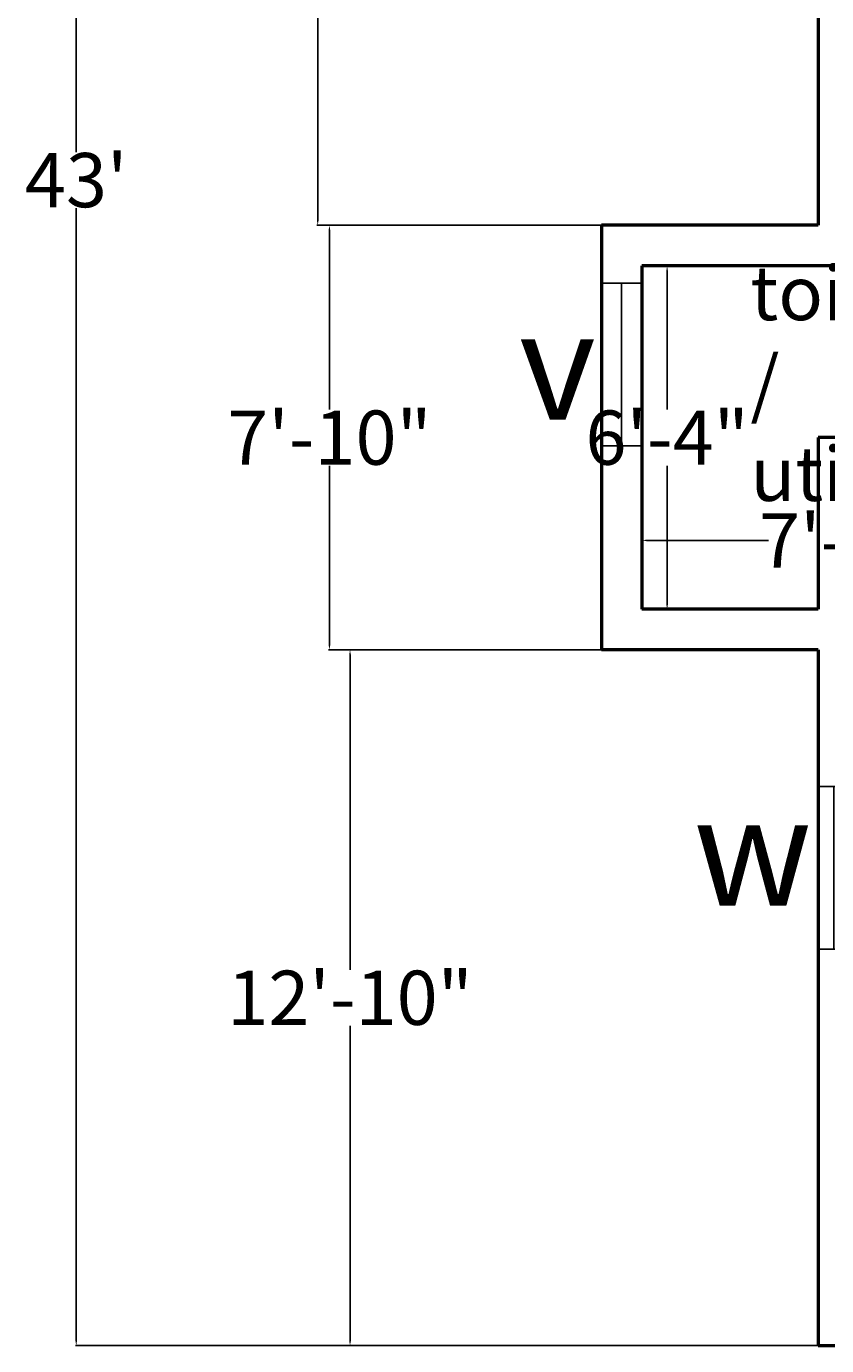
# Model space of a CAD drawing. Units: inches. Extents: x 409 to 7572, y 7 to 725.
# Tile 7 of 38: x 1521 to 1698, y 157 to 449. Entities that reach past the tile are written whole.
import ezdxf

# ---------------------------------------------------------------- set-up
doc = ezdxf.new("R2010")
doc.units = ezdxf.units.IN
doc.header["$MEASUREMENT"] = 0
for name, color, linetype, lineweight in [('A-ANNO-DIMS', 2, 'Continuous', 18), ('A-ANNO-SYMB', 3, 'Continuous', 25), ('A-AREA-IDEN', 7, 'Continuous', 25), ('A-GLAZ', 4, 'Continuous', 25), ('A-WALL', 7, 'Continuous', 50)]:
    doc.layers.add(name, color=color, linetype=linetype, lineweight=lineweight)
doc.styles.get("Standard").update_dxf_attribs({"font": 'arial.ttf'})
doc.dimstyles.get("Standard").update_dxf_attribs({"dimtxt": 2, "dimasz": 1, "dimexe": 0.18, "dimexo": 0.0625, "dimgap": 0.09, "dimtad": 0, "dimtih": 1, "dimtoh": 1, "dimdec": 0, "dimzin": 0, "dimdsep": 46, "dimlunit": 3, "dimtxsty": 'Standard', "dimcen": 0.09, "dimadec": 0, "dimazin": 0, "dimtfac": 1, "dimtdec": 0, "dimtofl": 0, "dimtmove": 0, "dimatfit": 3, "dimfxl": 1, "dimtolj": 1, "dimtzin": 0, "dimarcsym": 0})

# ---------------------------------------------------------------- blocks, each defined once
blk = doc.blocks.new('*D59')
at = {"layer": 'A-ANNO-DIMS', "color": 0, "lineweight": -2, "transparency": 16777216}
for p, q in [((1666.52, 395.53), (1662.7, 395.53)), ((1662.88, 394.53), (1662.88, 363.75)), ((1662.88, 320.53), (1662.88, 351.31)), ((1666.52, 319.53), (1662.7, 319.53))]:
    blk.add_line(p, q, dxfattribs=at)
at = {"layer": 'A-ANNO-DIMS', "color": 0, "transparency": 16777216}
for points in [[(1662.71, 394.53), (1663.05, 394.53), (1662.88, 395.53)], [(1662.71, 320.53), (1663.05, 320.53), (1662.88, 319.53)]]:
    blk.add_solid(points, dxfattribs=at)
at = {"layer": 'DEFPOINTS', "color": 0, "transparency": 16777216}
for p in [(1666.58, 395.53), (1662.88, 319.53), (1666.58, 319.53)]:
    blk.add_point(p, dxfattribs=at)
at = {"layer": 'A-ANNO-DIMS', "color": 0, "transparency": 16777216, "insert": (1662.88, 357.53), "char_height": 2, "attachment_point": 5}
blk.add_mtext('\\A1;{\\H6x;6\'-4"}', dxfattribs=at)
blk = doc.blocks.new('*D61')
at = {"layer": 'A-ANNO-DIMS', "color": 0, "lineweight": -2, "transparency": 16777216}
for p, q in [((1657.32, 346.33), (1657.32, 334.6)), ((1745.32, 346.33), (1745.32, 334.6)), ((1658.32, 334.78), (1685.33, 334.78)), ((1744.32, 334.78), (1717.31, 334.78))]:
    blk.add_line(p, q, dxfattribs=at)
at = {"layer": 'A-ANNO-DIMS', "color": 0, "transparency": 16777216}
for points in [[(1658.32, 334.95), (1658.32, 334.61), (1657.32, 334.78)], [(1744.32, 334.95), (1744.32, 334.61), (1745.32, 334.78)]]:
    blk.add_solid(points, dxfattribs=at)
at = {"layer": 'DEFPOINTS', "color": 0, "transparency": 16777216}
for p in [(1657.32, 346.39), (1745.32, 346.39), (1745.32, 334.78)]:
    blk.add_point(p, dxfattribs=at)
at = {"layer": 'A-ANNO-DIMS', "color": 0, "transparency": 16777216, "insert": (1701.32, 334.78), "char_height": 2, "attachment_point": 5}
blk.add_mtext('\\A1;{\\H6x;7\'-4"}', dxfattribs=at)
blk = doc.blocks.new('*D48')
at = {"layer": 'A-ANNO-DIMS', "color": 0, "lineweight": -2, "transparency": 16777216}
for p, q in [((1696.26, 672.53), (1585.36, 672.53)), ((1585.54, 671.53), (1585.54, 544.65)), ((1585.54, 405.53), (1585.54, 532.42)), ((1696.26, 404.53), (1585.36, 404.53))]:
    blk.add_line(p, q, dxfattribs=at)
at = {"layer": 'A-ANNO-DIMS', "color": 0, "transparency": 16777216}
for points in [[(1585.37, 671.53), (1585.71, 671.53), (1585.54, 672.53)], [(1585.37, 405.53), (1585.71, 405.53), (1585.54, 404.53)]]:
    blk.add_solid(points, dxfattribs=at)
at = {"layer": 'DEFPOINTS', "color": 0, "transparency": 16777216}
for p in [(1696.32, 672.53), (1585.54, 404.53), (1696.32, 404.53)]:
    blk.add_point(p, dxfattribs=at)
at = {"layer": 'A-ANNO-DIMS', "color": 0, "transparency": 16777216, "insert": (1585.54, 538.53), "char_height": 2, "attachment_point": 5}
blk.add_mtext('\\A1;{\\H6x;22\'-4"}', dxfattribs=at)
blk = doc.blocks.new('*D49')
at = {"layer": 'A-ANNO-DIMS', "color": 0, "lineweight": -2, "transparency": 16777216}
for p, q in [((1648.26, 404.53), (1587.95, 404.53)), ((1588.13, 403.53), (1588.13, 363.75)), ((1588.13, 311.53), (1588.13, 351.31)), ((1648.26, 310.53), (1587.95, 310.53))]:
    blk.add_line(p, q, dxfattribs=at)
at = {"layer": 'A-ANNO-DIMS', "color": 0, "transparency": 16777216}
for points in [[(1587.96, 403.53), (1588.29, 403.53), (1588.13, 404.53)], [(1587.96, 311.53), (1588.29, 311.53), (1588.13, 310.53)]]:
    blk.add_solid(points, dxfattribs=at)
at = {"layer": 'DEFPOINTS', "color": 0, "transparency": 16777216}
for p in [(1648.32, 404.53), (1588.13, 310.53), (1648.32, 310.53)]:
    blk.add_point(p, dxfattribs=at)
at = {"layer": 'A-ANNO-DIMS', "color": 0, "transparency": 16777216, "insert": (1588.13, 357.53), "char_height": 2, "attachment_point": 5}
blk.add_mtext('\\A1;{\\H6x;7\'-10"}', dxfattribs=at)
blk = doc.blocks.new('*D50')
at = {"layer": 'A-ANNO-DIMS', "color": 0, "lineweight": -2, "transparency": 16777216}
for p, q in [((1696.26, 310.53), (1592.51, 310.53)), ((1592.69, 309.53), (1592.69, 239.75)), ((1592.69, 157.53), (1592.69, 227.31)), ((1696.26, 156.53), (1592.51, 156.53))]:
    blk.add_line(p, q, dxfattribs=at)
at = {"layer": 'A-ANNO-DIMS', "color": 0, "transparency": 16777216}
for points in [[(1592.52, 309.53), (1592.86, 309.53), (1592.69, 310.53)], [(1592.52, 157.53), (1592.86, 157.53), (1592.69, 156.53)]]:
    blk.add_solid(points, dxfattribs=at)
at = {"layer": 'DEFPOINTS', "color": 0, "transparency": 16777216}
for p in [(1696.32, 310.53), (1592.69, 156.53), (1696.32, 156.53)]:
    blk.add_point(p, dxfattribs=at)
at = {"layer": 'A-ANNO-DIMS', "color": 0, "transparency": 16777216, "insert": (1592.69, 233.53), "char_height": 2, "attachment_point": 5}
blk.add_mtext('\\A1;{\\H6x;12\'-10"}', dxfattribs=at)
blk = doc.blocks.new('*D37')
at = {"layer": 'A-ANNO-DIMS', "color": 0, "lineweight": -2, "transparency": 16777216}
for p, q in [((1696.26, 672.53), (1531.9, 672.53)), ((1532.08, 671.53), (1532.08, 420.75)), ((1532.08, 157.53), (1532.08, 408.31)), ((1696.26, 156.53), (1531.9, 156.53))]:
    blk.add_line(p, q, dxfattribs=at)
at = {"layer": 'A-ANNO-DIMS', "color": 0, "transparency": 16777216}
for points in [[(1531.91, 671.53), (1532.25, 671.53), (1532.08, 672.53)], [(1531.91, 157.53), (1532.25, 157.53), (1532.08, 156.53)]]:
    blk.add_solid(points, dxfattribs=at)
at = {"layer": 'DEFPOINTS', "color": 0, "transparency": 16777216}
for p in [(1696.32, 672.53), (1532.08, 156.53), (1696.32, 156.53)]:
    blk.add_point(p, dxfattribs=at)
at = {"layer": 'A-ANNO-DIMS', "color": 0, "transparency": 16777216, "insert": (1532.08, 414.53), "char_height": 2, "attachment_point": 5}
blk.add_mtext("\\A1;{\\H6x;43'}", dxfattribs=at)
blk = doc.blocks.new('WIN-36')
for p, q in [((1699.82, 514.65), (1699.82, 478.65)), ((1700.82, 514.65), (1700.82, 478.65)), ((1701.82, 514.65), (1701.82, 478.65))]:
    blk.add_line(p, q)
blk.add_lwpolyline([(1705.32, 514.65), (1705.32, 478.65), (1696.32, 478.65), (1696.32, 514.65)], close=True)
blk = doc.blocks.new('VENT-36')
blk.add_line((5633.28, 355.73), (5633.28, 391.73))
blk.add_lwpolyline([(5628.78, 355.73), (5628.78, 391.73), (5637.78, 391.73), (5637.78, 355.73)], close=True)

msp = doc.modelspace()

# ---------------------------------------------------------------- linework, layer by layer
at = {"layer": 'A-WALL'}
for p, q in [((1696.32, 672.53), (1696.32, 404.53)), ((1696.32, 404.53), (1648.32, 404.53)), ((1648.32, 404.53), (1648.32, 310.53)), ((1705.32, 395.53), (1657.32, 395.53)), ((1657.32, 395.53), (1657.32, 319.53)), ((1696.32, 357.53), (1696.32, 319.53)), ((1705.32, 357.53), (1696.32, 357.53)), ((1696.32, 319.53), (1657.32, 319.53)), ((1696.32, 310.53), (1648.32, 310.53)), ((1696.32, 310.53), (1696.32, 156.53)), ((1696.32, 156.53), (2070.32, 156.53))]:
    msp.add_line(p, q, dxfattribs=at)

# ---------------------------------------------------------------- block references
at = {"layer": 'A-GLAZ'}
for name, p in [('VENT-36', (-3980.46, 0)), ('WIN-36', (0, -234.38))]:
    msp.add_blockref(name, p, dxfattribs=at)

# ---------------------------------------------------------------- texts
at = {"layer": 'A-ANNO-SYMB', "char_height": 24, "attachment_point": 1}
for s, insert in [('v', (1630.06, 385.54)), ('w', (1668.69, 277.95))]:
    msp.add_mtext_dynamic_manual_height_columns(s, width=18.2582, gutter_width=1, heights=[0], dxfattribs=dict(at, insert=insert))
at = {"layer": 'A-AREA-IDEN', "insert": (1681.32, 395.53), "char_height": 12, "attachment_point": 1}
msp.add_mtext_dynamic_manual_height_columns('toilet / utility', width=49.2946, gutter_width=1, heights=[0], dxfattribs=at)

# ---------------------------------------------------------------- dimensions: what is measured, and where the dimension line sits
at = {"layer": 'A-ANNO-DIMS'}
for base, p1, p2, picture, middle in [((1532.08, 156.53), (1696.32, 672.53), (1696.32, 156.53), '*D37', (1532.08, 414.53)), ((1585.54, 404.53), (1696.32, 672.53), (1696.32, 404.53), '*D48', (1585.54, 538.53)), ((1588.13, 310.53), (1648.32, 404.53), (1648.32, 310.53), '*D49', (1588.13, 357.53)), ((1662.88, 319.53), (1666.58, 395.53), (1666.58, 319.53), '*D59', (1662.88, 357.53)), ((1592.69, 156.53), (1696.32, 310.53), (1696.32, 156.53), '*D50', (1592.69, 233.53))]:
    dim = msp.add_linear_dim(base=base, p1=p1, p2=p2, angle=90, text='{\\H6x;<>}', dimstyle='Standard', override={"dimclrd": 0, "dimclre": 0, "dimclrt": 0}, dxfattribs=at)
    dim.commit()
    dim.dimension.update_dxf_attribs({"geometry": picture, "text_midpoint": middle})
dim = msp.add_linear_dim(base=(1745.32, 334.78), p1=(1657.32, 346.39), p2=(1745.32, 346.39), text='{\\H6x;<>}', dimstyle='Standard', override={"dimclrd": 0, "dimclre": 0, "dimclrt": 0}, dxfattribs=at)
dim.commit()
dim.dimension.update_dxf_attribs({"geometry": '*D61', "text_midpoint": (1701.32, 334.78)})

doc.saveas('drawing.dxf')
